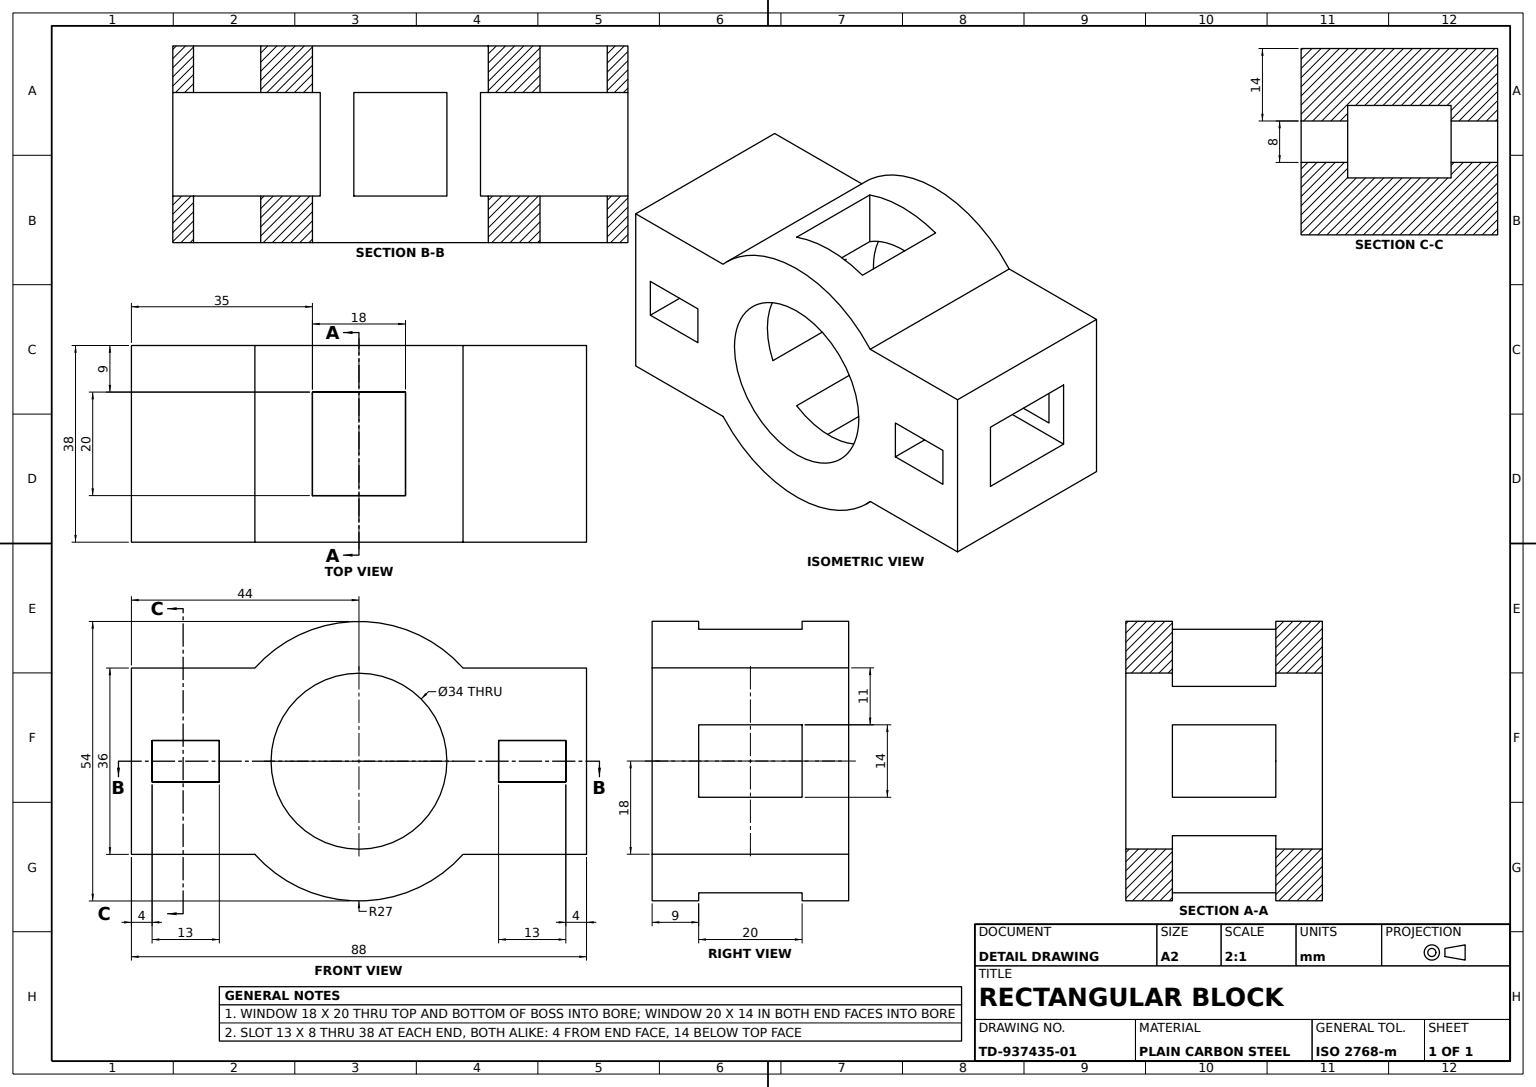
from build123d import *

# Parameters (mm, degrees)
BODY_PROFILE_SKETCH_R       = 17
BODY_PROFILE_SKETCH_W       = 13
BODY_PROFILE_SKETCH_H       = 8
BODY_EXTRUDE_38MM_DEPTH     = 38
WINDOW_CUT_20X14_DEPTH      = 100.584135283
WINDOW_CUT_20X14_DEPTH_BACK = 100.584135283
WINDOW_20X14_SKETCH_W       = 20
WINDOW_20X14_SKETCH_H       = 14
WINDOW_CUT_18X20_DEPTH      = 74.518705103
WINDOW_CUT_18X20_DEPTH_BACK = 74.518705103
WINDOW_18X20_SKETCH_W       = 18
WINDOW_18X20_SKETCH_H       = 20


with BuildPart() as part:
    # Body Profile Sketch → Body Extrude 38mm (new body)
    with BuildSketch(Plane.XY):
        with BuildLine():
            Line((-44, -18), (-20.124611797, -18))
            ThreePointArc((-20.124611797, -18), (0, -27), (20.124611797, -18))
            Line((20.124611797, -18), (44, -18))
            Line((44, -18), (44, 18))
            Line((44, 18), (20.124611797, 18))
            ThreePointArc((20.124611797, 18), (0, 27), (-20.124611797, 18))
            Line((-20.124611797, 18), (-44, 18))
            Line((-44, 18), (-44, -18))
        make_face()
        Circle(BODY_PROFILE_SKETCH_R, mode=Mode.SUBTRACT)
        with Locations((-33.5, 0)):
            Rectangle(BODY_PROFILE_SKETCH_W, BODY_PROFILE_SKETCH_H, mode=Mode.SUBTRACT)
        with Locations((33.5, 0)):
            Rectangle(BODY_PROFILE_SKETCH_W, BODY_PROFILE_SKETCH_H, mode=Mode.SUBTRACT)
    extrude(amount=-BODY_EXTRUDE_38MM_DEPTH)

    # Window 20x14 Sketch → Window Cut 20x14 (cut, two sides: drawn at the far end of the back side and taken through both)
    with BuildSketch(Plane.ZY.offset(44).offset(-WINDOW_CUT_20X14_DEPTH_BACK)):
        with Locations((-19, 0)):
            Rectangle(WINDOW_20X14_SKETCH_W, WINDOW_20X14_SKETCH_H)
    extrude(amount=WINDOW_CUT_20X14_DEPTH + WINDOW_CUT_20X14_DEPTH_BACK, mode=Mode.SUBTRACT)

    # Window 18x20 Sketch → Window Cut 18x20 (cut, two sides: drawn at the far end of the back side and taken through both)
    with BuildSketch(Plane(origin=(0, 18, 0), x_dir=(1, 0, 0), z_dir=(0, 1, 0)).offset(-WINDOW_CUT_18X20_DEPTH_BACK)):
        with Locations((0, 19)):
            Rectangle(WINDOW_18X20_SKETCH_W, WINDOW_18X20_SKETCH_H)
    extrude(amount=WINDOW_CUT_18X20_DEPTH + WINDOW_CUT_18X20_DEPTH_BACK, mode=Mode.SUBTRACT)


solid = part.part
